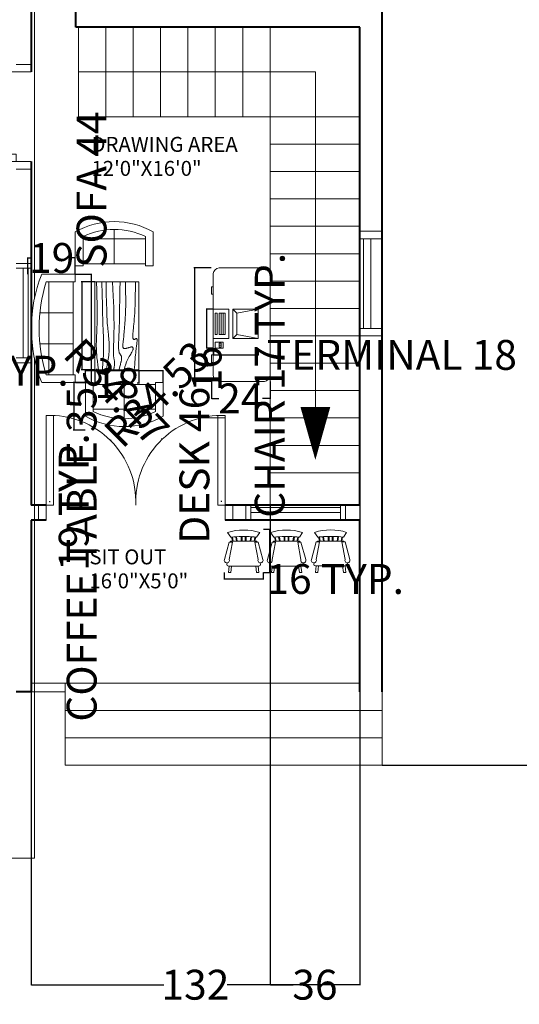
# Model space of a CAD drawing. Units: inches. Extents: x -101 to 786, y 26 to 880.
# Tile 2 of 9: x 178 to 379, y 26 to 422. Entities that reach past the tile are written whole.
import ezdxf

# ---------------------------------------------------------------- set-up
doc = ezdxf.new("R2010")
doc.units = ezdxf.units.IN
doc.header["$MEASUREMENT"] = 0
for name, color, linetype, lineweight in [('A-ANNO-DIMS', 2, 'Continuous', 18), ('A-ANNO-SYMB', 2, 'Continuous', 18), ('A-AREA-IDEN', 7, 'Continuous', 18), ('A-DOOR', 4, 'Continuous', 20), ('A-EQPM', 8, 'Continuous', 13), ('A-FLOR-STRS', 7, 'Continuous', 20), ('A-FURN', 8, 'Continuous', 13), ('A-GLAZ', 4, 'Continuous', 18), ('A-WALL', 7, 'Continuous', 40)]:
    doc.layers.add(name, color=color, linetype=linetype, lineweight=lineweight)
doc.styles.get("Standard").update_dxf_attribs({"font": 'arial.ttf'})
doc.dimstyles.get("Standard").update_dxf_attribs({"dimtxt": 12, "dimasz": 0.18, "dimexe": 0.18, "dimexo": 0.0625, "dimgap": 0.09, "dimtad": 0, "dimdec": 1, "dimzin": 0, "dimdsep": 46, "dimlunit": 3, "dimtxsty": 'Standard', "dimcen": 0.09, "dimadec": 0, "dimazin": 0, "dimtfac": 1, "dimtdec": 1, "dimtofl": 0, "dimtmove": 0, "dimatfit": 3, "dimfxl": 1, "dimtolj": 1, "dimtzin": 0, "dimarcsym": 0})

# ---------------------------------------------------------------- blocks, each defined once
blk = doc.blocks.new('Desk - 30 x 60 in.')
for p, q in [((-26.999995, 0), (26.999995, 0)), ((-29.999995, -27), (-29.999995, -3)), ((29.999995, -3), (29.999995, -27)), ((26.999995, -30), (-26.999995, -30)), ((-20.000005, -30), (-20.000005, -31)), ((-20.000005, -31), (-16.000005, -31)), ((-16.000005, -31), (-16.000005, -30)), ((15.999995, -31), (15.999995, -30)), ((19.999995, -31), (15.999995, -31)), ((19.999995, -30), (19.999995, -31))]:
    blk.add_line(p, q)
for centre, start, end in [((-26.499995, -3.5), 98.1301, 171.8699), ((26.499995, -3.5), 8.130102, 81.8699), ((-26.499995, -26.5), 188.1301, 261.8699), ((26.499995, -26.5), 278.1301, 351.8699)]:
    blk.add_arc(centre, 3.535534, start, end)
blk = doc.blocks.new('Sofa - Roundback 7 ft.')
for p, q in [((-12.00002, -32.4421), (-12.00003, -6.5971)), ((11.99997, -32.4421), (11.99998, -6.5971)), ((-36.000027, -34), (-36.000027, -11.4696)), ((-35.999844, -13.3819), (35.9998, -13.3819)), ((35.99998, -34), (35.99998, -11.4696)), ((-36.000027, -32.4421), (35.99998, -32.4421))]:
    blk.add_line(p, q)
for points in [[(-36.000027, -34), (-42.000027, -34), (-42.000027, -8)], [(41.99998, -8), (41.99998, -34), (35.99998, -34)]]:
    blk.add_lwpolyline(points)
for centre, radius, start, end in [((0, -114.25), 114.25, 68.43141, 111.5686), ((-0.00001, -127.1968), 121.1968, 72.72033, 107.2797)]:
    blk.add_arc(centre, radius, start, end)
blk = doc.blocks.new('Sofa - Roundback Loveseat 5 ft.')
for p, q in [((0, -32.44198), (0, -5.99998)), ((-24, -33.99998), (-24, -11.46958)), ((-23.9998, -13.38178), (23.99986, -13.38178)), ((24.00004, -33.99998), (24.00004, -11.46958)), ((-24, -32.44198), (24.00004, -32.44198))]:
    blk.add_line(p, q)
for points in [[(-24, -33.99998), (-30, -33.99998), (-30, -7.99998)], [(30.00004, -7.99998), (30.00004, -33.99998), (24.00004, -33.99998)]]:
    blk.add_lwpolyline(points)
for centre, radius, start, end in [((0, -60.24998), 60.24998, 60.13715, 119.8628), ((0, -61.38438), 55.38444, 64.32083, 115.6792)]:
    blk.add_arc(centre, radius, start, end)
blk = doc.blocks.new('Table - Rectangular Woodgrain 60 x 30 in.')
for p, q in [((0, 0), (0, -30)), ((60, 0), (0, 0)), ((60, -30), (60, 0)), ((0, -30), (60, -30))]:
    blk.add_line(p, q)
for points in [[(0, -2.4), (4.8155, -2.418), (9.0302, -2.4688), (12.709, -2.5477), (15.9167, -2.65), (18.7181, -2.7711), (21.1781, -2.9063), (23.3616, -3.0508), (25.3333, -3.2), (27.1477, -3.3495), (28.8172, -3.4958), (30.3437, -3.636), (31.7291, -3.7667), (32.9756, -3.8849), (34.0849, -3.9875), (35.059, -4.0714), (35.9, -4.1334), (36.6114, -4.1711), (37.2041, -4.1854), (37.6906, -4.1779), (38.0833, -4.15), (38.3948, -4.1034), (38.6375, -4.0396), (38.8239, -3.9602), (38.9666, -3.8667), (39.0764, -3.7608), (39.1573, -3.6448), (39.2116, -3.521), (39.2416, -3.3917), (39.2498, -3.2593), (39.2385, -3.1261), (39.21, -2.9944), (39.1666, -2.8667), (39.111, -2.7447), (39.0468, -2.6281), (38.978, -2.5163), (38.9083, -2.4083), (38.8418, -2.3035), (38.7823, -2.201), (38.7337, -2.1001), (38.7, -2), (38.6844, -1.9003), (38.6875, -1.8021), (38.7094, -1.707), (38.75, -1.6167), (38.8094, -1.5326), (38.8875, -1.4563), (38.9844, -1.3893), (39.1, -1.3333), (39.2351, -1.2896), (39.3937, -1.2583), (39.5804, -1.2396), (39.8, -1.2333), (40.057, -1.2396), (40.3562, -1.2583), (40.7023, -1.2896), (41.1, -1.3333), (41.5547, -1.3895), (42.0755, -1.4573), (42.6721, -1.5361), (43.3542, -1.625), (44.1316, -1.7233), (45.014, -1.8302), (46.0114, -1.9449), (47.1333, -2.0667), (48.3862, -2.1947), (49.7625, -2.3281), (51.2513, -2.4663), (52.8416, -2.6083), (54.5226, -2.7535), (56.2833, -2.9011), (58.1127, -3.0501), (60, -3.2)], [(0, -9.2), (6.5759, -9.0858), (11.9385, -9.0365), (16.2527, -9.0418), (19.6833, -9.0917), (22.3952, -9.1759), (24.5531, -9.2844), (26.322, -9.4069), (27.8666, -9.5333), (29.3241, -9.6553), (30.7203, -9.7719), (32.0532, -9.8837), (33.3208, -9.9917), (34.5213, -10.0965), (35.6526, -10.199), (36.7128, -10.2999), (37.7, -10.4), (38.6129, -10.4996), (39.4531, -10.5969), (40.223, -10.6895), (40.925, -10.775), (41.5613, -10.8512), (42.1344, -10.9156), (42.6465, -10.966), (43.1, -11), (43.4976, -11.0158), (43.8437, -11.0136), (44.143, -10.9942), (44.4, -10.9583), (44.6195, -10.9069), (44.8062, -10.8406), (44.9648, -10.7603), (45.1, -10.6667), (45.2155, -10.5598), (45.3114, -10.4365), (45.3871, -10.2929), (45.4416, -10.125), (45.4743, -9.929), (45.4844, -9.7011), (45.4709, -9.4371), (45.4333, -9.1333), (45.3716, -8.7883), (45.2896, -8.4104), (45.1919, -8.0107), (45.0833, -7.6), (44.9685, -7.1893), (44.8521, -6.7896), (44.7388, -6.4117), (44.6333, -6.0667), (44.54, -5.7628), (44.4614, -5.4979), (44.4001, -5.2675), (44.3583, -5.0667), (44.3384, -4.8909), (44.3427, -4.7354), (44.3736, -4.5956), (44.4333, -4.4667), (44.5236, -4.3453), (44.6427, -4.2333), (44.7884, -4.1339), (44.9583, -4.05), (45.1501, -3.9849), (45.3614, -3.9417), (45.59, -3.9234), (45.8333, -3.9333), (46.0915, -3.9749), (46.3734, -4.0531), (46.6906, -4.1736), (47.0542, -4.3417), (47.4756, -4.5629), (47.9661, -4.8427), (48.5372, -5.1866), (49.2, -5.6), (49.9676, -6.0844), (50.8594, -6.625), (51.8965, -7.2031), (53.1, -7.8), (54.491, -8.3969), (56.0906, -8.975), (57.9199, -9.5156), (60, -10)], [(0, -12.8), (5.1847, -12.9322), (9.6213, -13.0323), (13.3963, -13.1059), (16.5958, -13.1583), (19.3063, -13.1952), (21.614, -13.2219), (23.6054, -13.2439), (25.3666, -13.2667), (26.9728, -13.2947), (28.4531, -13.3281), (29.8256, -13.3663), (31.1083, -13.4083), (32.3191, -13.4535), (33.476, -13.501), (34.597, -13.5501), (35.7, -13.6), (36.7984, -13.6497), (37.8875, -13.6979), (38.9578, -13.743), (40, -13.7833), (41.0047, -13.8174), (41.9625, -13.8438), (42.864, -13.8607), (43.7, -13.8667), (44.4631, -13.8604), (45.1552, -13.8417), (45.7801, -13.8104), (46.3416, -13.7667), (46.8439, -13.7104), (47.2906, -13.6417), (47.6858, -13.5604), (48.0333, -13.4667), (48.3375, -13.3608), (48.6042, -13.2448), (48.8396, -13.121), (49.05, -12.9917), (49.2417, -12.8593), (49.4208, -12.7261), (49.5937, -12.5944), (49.7667, -12.4667), (49.9452, -12.3451), (50.1323, -12.2313), (50.3303, -12.1268), (50.5416, -12.0333), (50.7686, -11.9524), (51.0135, -11.8854), (51.2788, -11.8341), (51.5666, -11.8), (51.8785, -11.7843), (52.2116, -11.7865), (52.562, -11.8059), (52.926, -11.8417), (53.2998, -11.8931), (53.6795, -11.9594), (54.0614, -12.0397), (54.4416, -12.1333), (54.8223, -12.2401), (55.2293, -12.3625), (55.6942, -12.5037), (56.2489, -12.6667), (56.9251, -12.8547), (57.7545, -13.0708), (58.7689, -13.3182), (60, -13.6)], [(0, -18), (5.124, -17.7273), (9.6609, -17.5057), (13.6705, -17.3303), (17.2125, -17.1958), (20.3467, -17.0973), (23.1328, -17.0297), (25.6307, -16.9878), (27.9, -16.9667), (29.9928, -16.9617), (31.9302, -16.9703), (33.7254, -16.9907), (35.3917, -17.0208), (36.9423, -17.0588), (38.3906, -17.1026), (39.7499, -17.1503), (41.0333, -17.2), (42.2519, -17.2496), (43.4073, -17.2969), (44.4986, -17.3395), (45.525, -17.375), (46.4858, -17.4012), (47.3802, -17.4156), (48.2074, -17.416), (48.9667, -17.4), (49.6583, -17.3662), (50.2872, -17.3167), (50.8595, -17.2547), (51.3812, -17.1833), (51.8584, -17.1057), (52.2971, -17.025), (52.7034, -16.9443), (53.0833, -16.8667), (53.443, -16.7951), (53.789, -16.7313), (54.128, -16.6768), (54.4666, -16.6334), (54.8115, -16.6024), (55.1693, -16.5854), (55.5465, -16.5841), (55.95, -16.6), (56.3828, -16.6337), (56.8346, -16.6823), (57.2915, -16.7418), (57.7396, -16.8084), (58.165, -16.878), (58.5539, -16.9469), (58.8924, -17.0111), (59.1666, -17.0667), (59.3679, -17.1107), (59.5078, -17.1438), (59.6032, -17.1675), (59.6708, -17.1833), (59.7275, -17.193), (59.7901, -17.1979), (59.8753, -17.1998), (60, -17.2)], [(0, -22.4), (8.0098, -22.2501), (14.4094, -22.1011), (19.4168, -21.9535), (23.25, -21.8083), (26.1269, -21.6663), (28.2656, -21.5281), (29.884, -21.3947), (31.2, -21.2667), (32.3967, -21.1448), (33.5172, -21.0292), (34.5697, -20.9198), (35.5625, -20.8167), (36.5037, -20.7198), (37.4015, -20.6292), (38.2642, -20.5448), (39.1, -20.4667), (39.9164, -20.3951), (40.7187, -20.3313), (41.5117, -20.2768), (42.3, -20.2333), (43.0883, -20.2024), (43.8812, -20.1854), (44.6836, -20.1841), (45.5, -20.2), (46.3328, -20.234), (47.1747, -20.2844), (48.0163, -20.3488), (48.8479, -20.425), (49.66, -20.5106), (50.4429, -20.6031), (51.1872, -20.7004), (51.8833, -20.8), (52.5246, -20.8999), (53.1166, -20.9995), (53.6681, -21.0983), (54.1875, -21.1958), (54.6834, -21.2919), (55.1646, -21.3859), (55.6394, -21.4777), (56.1167, -21.5667), (56.6028, -21.6515), (57.0961, -21.7266), (57.5929, -21.7852), (58.0896, -21.8208), (58.5823, -21.8268), (59.0674, -21.7964), (59.5412, -21.723), (60, -21.6)], [(0, -25.2), (8.6355, -25.0504), (15.7026, -24.9031), (21.4049, -24.7606), (25.9458, -24.625), (29.529, -24.4988), (32.3578, -24.3844), (34.6359, -24.284), (36.5667, -24.2), (38.3213, -24.1341), (39.9417, -24.0854), (41.437, -24.0523), (42.8167, -24.0333), (44.0901, -24.0268), (45.2667, -24.0313), (46.3557, -24.0451), (47.3667, -24.0667), (48.309, -24.0947), (49.1928, -24.1287), (50.0284, -24.168), (50.826, -24.2125), (51.5959, -24.2617), (52.3483, -24.3151), (53.0935, -24.3725), (53.8417, -24.4334), (54.6009, -24.497), (55.3699, -24.561), (56.1454, -24.6226), (56.9239, -24.6792), (57.7021, -24.7279), (58.4764, -24.7662), (59.2435, -24.7911), (60, -24.8)], [(0, -28.8), (5.6867, -28.6681), (10.45, -28.5698), (14.407, -28.5012), (17.675, -28.4584), (20.3711, -28.4374), (22.6125, -28.4344), (24.5164, -28.4455), (26.2, -28.4667), (27.762, -28.4947), (29.2276, -28.5281), (30.6033, -28.5663), (31.8958, -28.6084), (33.1118, -28.6535), (34.2578, -28.7011), (35.3405, -28.7501), (36.3666, -28.8), (37.3443, -28.8497), (38.288, -28.8974), (39.2137, -28.9412), (40.1375, -28.9792), (41.0753, -29.0093), (42.0432, -29.0297), (43.0572, -29.0384), (44.1333, -29.0333), (45.2936, -29.0114), (46.5843, -28.9641), (48.0579, -28.8816), (49.7666, -28.7542), (51.7629, -28.5721), (54.0989, -28.3255), (56.8272, -28.0048), (60, -27.6)]]:
    blk.add_lwpolyline(points)
blk = doc.blocks.new('Computer Terminal')
for p, q in [((-10, 11.5), (5, 11.5)), ((-8, 0.5), (-10, 11.5)), ((-10, -1.5), (-10, 11.5)), ((5, 11.5), (3, 0.5)), ((5, 11.5), (5, -1.5)), ((-10, -1.5), (-8, 0.5)), ((3, 0.5), (-8, 0.5)), ((3, 0.5), (5, -1.5)), ((5, -1.5), (-10, -1.5)), ((-10, -11.5), (-10, -3.5)), ((-10, -3.5), (5, -3.5)), ((5, -3.5), (5, -11.5)), ((-8, -5.5), (-8, -8.5)), ((3, -5.5), (-8, -5.5)), ((3, -6.5), (-8, -6.5)), ((-8, -7.5), (3, -7.5)), ((-8, -8.5), (3, -8.5)), ((-8, -9.5), (-8, -10.5)), ((3, -9.5), (-8, -9.5)), ((3, -8.5), (3, -5.5)), ((3, -10.5), (3, -9.5)), ((10, -6.5), (7, -6.5)), ((7, -6.5), (7, -10.5)), ((9.5, -7.5), (7.5, -7.5)), ((7.5, -7.5), (7.5, -8.5)), ((7.5, -8.5), (9.5, -8.5)), ((8.5, -7.5), (8.5, -8.5)), ((9.5, -8.5), (9.5, -7.5)), ((10, -10.5), (10, -6.5)), ((5, -11.5), (-10, -11.5)), ((-8, -10.5), (3, -10.5)), ((7, -10.5), (10, -10.5))]:
    blk.add_line(p, q)
blk = doc.blocks.new('Chair - Rocking')
for p, q in [((-8, -4.5), (-10, -1.5)), ((-7.5, -4.5), (-7, -7)), ((-6.5, -7), (-7.02225, -4.43)), ((-4.5, -7), (-4.96674, -4.19951)), ((-4, -7), (-4.40532, -4.16272)), ((-1.5, -4.05012), (-1.5, -7)), ((-1, -7), (-1, -4.05012)), ((1, -7), (1, -4.04655)), ((1.5, -4.05012), (1.5, -7)), ((4, -7), (4.40187, -4.18694)), ((4.5, -7), (4.96761, -4.19437)), ((6.5, -7), (7, -4.4057)), ((7.5, -4.5), (7, -7)), ((8, -4.5), (10, -1.5)), ((-9, -7.5), (-12, -18.49999)), ((-7, -7.5), (-9, -7.5)), ((-9, -18.49999), (-7, -7.5)), ((-8.23428, -6.99939), (-8.3093, -7.47958)), ((-8.23041, -7), (8.23915, -7)), ((7, -7.5), (9, -7.5)), ((9, -18.49999), (7, -7.5)), ((8.31071, -7.48854), (8.23449, -7.00073)), ((9, -7.5), (12, -18.49999)), ((-10.36644, -20.64523), (-10.5, -21.49999)), ((-9, -22.49999), (-9.5, -26.49999)), ((0, -22.49999), (-9.5, -22.49999)), ((-8, -26.49999), (-7.5, -22.49999)), ((0, -22.49999), (9.5, -22.49999)), ((8, -26.49999), (7.5, -22.49999)), ((9, -22.49999), (9.5, -26.49999)), ((10.5, -21.49999), (10.3575, -20.58798)), ((-9.5, -26.49999), (-8, -26.49999)), ((9.5, -26.49999), (8, -26.49999))]:
    blk.add_line(p, q)
for centre, radius, start, end in [((0, -34.08333), 34.08333, 72.93847, 107.0615), ((0, -68.25004), 64.25, 93.92211, 97.15267), ((0, -68.25004), 64.25, 82.84733, 93.92211), ((-10.5, -18.99999), 1.58114, 161.5651, 18.43495), ((-9.5, -21.49999), 1, 180, 270), ((10.5, -18.99999), 1.58114, 161.5651, 18.43495), ((9.5, -21.49999), 1, 270, 0)]:
    blk.add_arc(centre, radius, start, end)
blk = doc.blocks.new('DOOR-SINGLE-36')
for p, q in [((-39, 0), (-39, -6)), ((-36, 0), (-36, -6)), ((0, 0), (0, -6)), ((3, 0), (3, -6))]:
    blk.add_line(p, q)
blk.add_lwpolyline([(0, 0), (-3, 0), (-3, 36), (0, 36)], close=True)
blk.add_arc((-1.5, 1.5), 34.53, 87.5104, 182.4896)
blk = doc.blocks.new('WIN-36-WALL9')
for p, q in [((0, 42), (9, 42)), ((0, 39), (9, 39)), ((1.5, 39), (1.5, 3)), ((4.5, 39), (4.5, 3)), ((9, 3), (0, 3)), ((9, 0), (0, 0))]:
    blk.add_line(p, q)
blk = doc.blocks.new('*D29')
at = {"layer": 'A-ANNO-DIMS', "color": 0, "lineweight": -2, "transparency": 16777216}
for p, q in [((275.82, 217.12), (278.54, 217.12)), ((278.36, 217.12), (278.36, 217.3)), ((278.36, 199.92), (278.36, 216.94)), ((275.82, 199.74), (278.54, 199.74))]:
    blk.add_line(p, q, dxfattribs=at)
at = {"layer": 'A-ANNO-DIMS', "color": 0, "transparency": 16777216}
for points in [[(278.33, 216.94), (278.39, 216.94), (278.36, 217.12)], [(278.33, 199.92), (278.39, 199.92), (278.36, 199.74)]]:
    blk.add_solid(points, dxfattribs=at)
at = {"layer": 'Defpoints', "color": 0, "transparency": 16777216}
for p in [(275.76, 217.12), (278.36, 217.12), (275.76, 199.74)]:
    blk.add_point(p, dxfattribs=at)
at = {"layer": 'A-ANNO-DIMS', "color": 0, "transparency": 16777216, "insert": (278.36, 274.93), "char_height": 12, "attachment_point": 5, "rotation": 90}
blk.add_mtext('\\A1;CHAIR 17 TYP.', dxfattribs=at)
blk = doc.blocks.new('*D30')
at = {"layer": 'A-ANNO-DIMS', "color": 0, "lineweight": -2, "transparency": 16777216}
for p, q in [((260.03, 199.68), (260.03, 196.96)), ((275.76, 199.68), (275.76, 196.96)), ((260.21, 197.14), (275.58, 197.14)), ((275.76, 197.14), (275.94, 197.14))]:
    blk.add_line(p, q, dxfattribs=at)
at = {"layer": 'A-ANNO-DIMS', "color": 0, "transparency": 16777216}
for points in [[(260.21, 197.17), (260.21, 197.11), (260.03, 197.14)], [(275.58, 197.17), (275.58, 197.11), (275.76, 197.14)]]:
    blk.add_solid(points, dxfattribs=at)
at = {"layer": 'Defpoints', "color": 0, "transparency": 16777216}
for p in [(260.03, 199.74), (275.76, 199.74), (275.76, 197.14)]:
    blk.add_point(p, dxfattribs=at)
at = {"layer": 'A-ANNO-DIMS', "color": 0, "transparency": 16777216, "insert": (304.67, 197.14), "char_height": 12, "attachment_point": 5}
blk.add_mtext('\\A1;16 TYP.', dxfattribs=at)
blk = doc.blocks.new('*D55')
at = {"layer": 'A-ANNO-DIMS', "color": 0, "lineweight": -2, "transparency": 16777216}
for p, q in [((204.29, 276.16), (204.29, 280.97)), ((235.59, 276.16), (235.59, 280.97)), ((204.29, 280.79), (204.11, 280.79)), ((235.41, 280.79), (204.47, 280.79))]:
    blk.add_line(p, q, dxfattribs=at)
at = {"layer": 'A-ANNO-DIMS', "color": 0, "transparency": 16777216}
for points in [[(204.47, 280.82), (204.47, 280.76), (204.29, 280.79)], [(235.41, 280.82), (235.41, 280.76), (235.59, 280.79)]]:
    blk.add_solid(points, dxfattribs=at)
at = {"layer": 'Defpoints', "color": 0, "transparency": 16777216}
for p in [(204.29, 280.79), (204.29, 276.1), (235.59, 276.1)]:
    blk.add_point(p, dxfattribs=at)
at = {"layer": 'A-ANNO-DIMS', "color": 0, "transparency": 16777216, "insert": (128.5, 280.79), "char_height": 12, "attachment_point": 5}
blk.add_mtext('\\A1;LOVESEAT 31 TYP.', dxfattribs=at)
blk = doc.blocks.new('*D56')
at = {"layer": 'A-ANNO-DIMS', "color": 0, "lineweight": -2, "transparency": 16777216}
for p, q in [((204.23, 276.1), (199.42, 276.1)), ((199.6, 275.92), (199.6, 257.15)), ((204.23, 256.97), (199.42, 256.97)), ((199.6, 256.97), (199.6, 256.79))]:
    blk.add_line(p, q, dxfattribs=at)
at = {"layer": 'A-ANNO-DIMS', "color": 0, "transparency": 16777216}
for points in [[(199.57, 275.92), (199.63, 275.92), (199.6, 276.1)], [(199.57, 257.15), (199.63, 257.15), (199.6, 256.97)]]:
    blk.add_solid(points, dxfattribs=at)
at = {"layer": 'Defpoints', "color": 0, "transparency": 16777216}
for p in [(204.29, 276.1), (199.6, 256.97), (204.29, 256.97)]:
    blk.add_point(p, dxfattribs=at)
at = {"layer": 'A-ANNO-DIMS', "color": 0, "transparency": 16777216, "insert": (199.6, 228.06), "char_height": 12, "attachment_point": 5, "rotation": 90}
blk.add_mtext('\\A1;19 TYP.', dxfattribs=at)
blk = doc.blocks.new('*D69')
at = {"layer": 'A-ANNO-DIMS', "color": 0, "lineweight": -2, "transparency": 16777216}
for p, q in [((254.88, 322.12), (247.93, 322.12)), ((248.11, 321.94), (248.11, 276.7)), ((254.88, 276.52), (247.93, 276.52)), ((248.11, 276.52), (248.11, 276.34))]:
    blk.add_line(p, q, dxfattribs=at)
at = {"layer": 'A-ANNO-DIMS', "color": 0, "transparency": 16777216}
for points in [[(248.08, 321.94), (248.14, 321.94), (248.11, 322.12)], [(248.08, 276.7), (248.14, 276.7), (248.11, 276.52)]]:
    blk.add_solid(points, dxfattribs=at)
at = {"layer": 'Defpoints', "color": 0, "transparency": 16777216}
for p in [(254.95, 322.12), (248.11, 276.52), (254.95, 276.52)]:
    blk.add_point(p, dxfattribs=at)
at = {"layer": 'A-ANNO-DIMS', "color": 0, "transparency": 16777216, "insert": (248.11, 242.81), "char_height": 12, "attachment_point": 5, "rotation": 90}
blk.add_mtext('\\A1;DESK 46', dxfattribs=at)
blk = doc.blocks.new('*D70')
at = {"layer": 'A-ANNO-DIMS', "color": 0, "lineweight": -2, "transparency": 16777216}
for p, q in [((254.95, 276.46), (254.95, 269.5)), ((278.51, 276.46), (278.51, 269.5)), ((255.13, 269.68), (257.96, 269.68)), ((278.33, 269.68), (275.49, 269.68))]:
    blk.add_line(p, q, dxfattribs=at)
at = {"layer": 'A-ANNO-DIMS', "color": 0, "transparency": 16777216}
for points in [[(255.13, 269.71), (255.13, 269.65), (254.95, 269.68)], [(278.33, 269.71), (278.33, 269.65), (278.51, 269.68)]]:
    blk.add_solid(points, dxfattribs=at)
at = {"layer": 'Defpoints', "color": 0, "transparency": 16777216}
for p in [(254.95, 276.52), (278.51, 276.52), (278.51, 269.68)]:
    blk.add_point(p, dxfattribs=at)
at = {"layer": 'A-ANNO-DIMS', "color": 0, "transparency": 16777216, "insert": (266.73, 269.68), "char_height": 12, "attachment_point": 5}
blk.add_mtext('\\A1;24', dxfattribs=at)
blk = doc.blocks.new('*D71')
at = {"layer": 'A-ANNO-DIMS', "color": 0, "lineweight": -2, "transparency": 16777216}
for p, q in [((200.31, 319.56), (206.96, 319.56)), ((206.78, 319.56), (206.78, 319.74)), ((206.78, 276.19), (206.78, 319.38)), ((200.31, 276.01), (206.96, 276.01))]:
    blk.add_line(p, q, dxfattribs=at)
at = {"layer": 'A-ANNO-DIMS', "color": 0, "transparency": 16777216}
for points in [[(206.75, 319.38), (206.81, 319.38), (206.78, 319.56)], [(206.75, 276.19), (206.81, 276.19), (206.78, 276.01)]]:
    blk.add_solid(points, dxfattribs=at)
at = {"layer": 'Defpoints', "color": 0, "transparency": 16777216}
for p in [(200.25, 319.56), (206.78, 319.56), (200.25, 276.01)]:
    blk.add_point(p, dxfattribs=at)
at = {"layer": 'A-ANNO-DIMS', "color": 0, "transparency": 16777216, "insert": (206.78, 353.52), "char_height": 12, "attachment_point": 5, "rotation": 90}
blk.add_mtext('\\A1;SOFA 44', dxfattribs=at)
blk = doc.blocks.new('*D72')
at = {"layer": 'A-ANNO-DIMS', "color": 0, "lineweight": -2, "transparency": 16777216}
for p, q in [((181.24, 319.62), (181.24, 326.27)), ((181.42, 326.09), (182.61, 326.09)), ((200.07, 326.09), (198.87, 326.09)), ((200.25, 319.62), (200.25, 326.27))]:
    blk.add_line(p, q, dxfattribs=at)
at = {"layer": 'A-ANNO-DIMS', "color": 0, "transparency": 16777216}
for points in [[(181.42, 326.12), (181.42, 326.06), (181.24, 326.09)], [(200.07, 326.12), (200.07, 326.06), (200.25, 326.09)]]:
    blk.add_solid(points, dxfattribs=at)
at = {"layer": 'Defpoints', "color": 0, "transparency": 16777216}
for p in [(181.24, 326.09), (181.24, 319.56), (200.25, 319.56)]:
    blk.add_point(p, dxfattribs=at)
at = {"layer": 'A-ANNO-DIMS', "color": 0, "transparency": 16777216, "insert": (190.74, 326.09), "char_height": 12, "attachment_point": 5}
blk.add_mtext('\\A1;19', dxfattribs=at)
blk = doc.blocks.new('*D73')
at = {"layer": 'A-ANNO-DIMS', "color": 0, "lineweight": -2, "transparency": 16777216}
for p, q in [((208.06, 316.53), (202.63, 316.53)), ((202.81, 316.35), (202.81, 281.31)), ((208.06, 281.13), (202.63, 281.13)), ((202.81, 281.13), (202.81, 280.95))]:
    blk.add_line(p, q, dxfattribs=at)
at = {"layer": 'A-ANNO-DIMS', "color": 0, "transparency": 16777216}
for points in [[(202.78, 316.35), (202.84, 316.35), (202.81, 316.53)], [(202.78, 281.31), (202.84, 281.31), (202.81, 281.13)]]:
    blk.add_solid(points, dxfattribs=at)
at = {"layer": 'Defpoints', "color": 0, "transparency": 16777216}
for p in [(208.12, 316.53), (202.81, 281.13), (208.12, 281.13)]:
    blk.add_point(p, dxfattribs=at)
at = {"layer": 'A-ANNO-DIMS', "color": 0, "transparency": 16777216, "insert": (202.81, 207.08), "char_height": 12, "attachment_point": 5, "rotation": 90}
blk.add_mtext('\\A1;COFFEE TABLE 35', dxfattribs=at)
blk = doc.blocks.new('*D74')
at = {"layer": 'A-ANNO-DIMS', "color": 0, "lineweight": -2, "transparency": 16777216}
for p, q in [((208.12, 281.06), (208.12, 275.64)), ((225.82, 281.06), (225.82, 275.64)), ((208.3, 275.82), (208.84, 275.82)), ((225.64, 275.82), (225.1, 275.82))]:
    blk.add_line(p, q, dxfattribs=at)
at = {"layer": 'A-ANNO-DIMS', "color": 0, "transparency": 16777216}
for points in [[(208.3, 275.85), (208.3, 275.79), (208.12, 275.82)], [(225.64, 275.85), (225.64, 275.79), (225.82, 275.82)]]:
    blk.add_solid(points, dxfattribs=at)
at = {"layer": 'Defpoints', "color": 0, "transparency": 16777216}
for p in [(208.12, 281.13), (225.82, 281.13), (225.82, 275.82)]:
    blk.add_point(p, dxfattribs=at)
at = {"layer": 'A-ANNO-DIMS', "color": 0, "transparency": 16777216, "insert": (216.97, 275.82), "char_height": 12, "attachment_point": 5}
blk.add_mtext('\\A1;18', dxfattribs=at)
blk = doc.blocks.new('*D75')
at = {"layer": 'A-ANNO-DIMS', "color": 0, "lineweight": -2, "transparency": 16777216}
for p, q in [((255.71, 289.78), (255.71, 286.97)), ((273.71, 289.78), (273.71, 286.97)), ((255.89, 287.15), (273.53, 287.15)), ((273.71, 287.15), (273.89, 287.15))]:
    blk.add_line(p, q, dxfattribs=at)
at = {"layer": 'A-ANNO-DIMS', "color": 0, "transparency": 16777216}
for points in [[(255.89, 287.18), (255.89, 287.12), (255.71, 287.15)], [(273.53, 287.18), (273.53, 287.12), (273.71, 287.15)]]:
    blk.add_solid(points, dxfattribs=at)
at = {"layer": 'Defpoints', "color": 0, "transparency": 16777216}
for p in [(255.71, 289.85), (273.71, 289.85), (273.71, 287.15)]:
    blk.add_point(p, dxfattribs=at)
at = {"layer": 'A-ANNO-DIMS', "color": 0, "transparency": 16777216, "insert": (327.45, 287.15), "char_height": 12, "attachment_point": 5}
blk.add_mtext('\\A1;TERMINAL 18', dxfattribs=at)
blk = doc.blocks.new('*D76')
at = {"layer": 'A-ANNO-DIMS', "color": 0, "lineweight": -2, "transparency": 16777216}
for p, q in [((255.64, 305.5), (252.83, 305.5)), ((253.01, 305.32), (253.01, 290.03)), ((255.64, 289.85), (252.83, 289.85)), ((253.01, 289.85), (253.01, 289.67))]:
    blk.add_line(p, q, dxfattribs=at)
at = {"layer": 'A-ANNO-DIMS', "color": 0, "transparency": 16777216}
for points in [[(252.98, 305.32), (253.04, 305.32), (253.01, 305.5)], [(252.98, 290.03), (253.04, 290.03), (253.01, 289.85)]]:
    blk.add_solid(points, dxfattribs=at)
at = {"layer": 'Defpoints', "color": 0, "transparency": 16777216}
for p in [(255.71, 305.5), (253.01, 289.85), (255.71, 289.85)]:
    blk.add_point(p, dxfattribs=at)
at = {"layer": 'A-ANNO-DIMS', "color": 0, "transparency": 16777216, "insert": (253.01, 281.55), "char_height": 12, "attachment_point": 5, "rotation": 90}
blk.add_mtext('\\A1;16', dxfattribs=at)
blk = doc.blocks.new('*D80')
at = {"layer": 'A-ANNO-DIMS', "color": 0, "lineweight": -2, "transparency": 16777216}
for p, q in [((323.57, 781.8), (424.94, 781.8)), ((424.76, 781.62), (424.76, 472.49)), ((424.76, 122.52), (424.76, 431.66)), ((323.57, 122.34), (424.94, 122.34))]:
    blk.add_line(p, q, dxfattribs=at)
at = {"layer": 'A-ANNO-DIMS', "color": 0, "transparency": 16777216}
for points in [[(424.73, 781.62), (424.79, 781.62), (424.76, 781.8)], [(424.73, 122.52), (424.79, 122.52), (424.76, 122.34)]]:
    blk.add_solid(points, dxfattribs=at)
at = {"layer": 'Defpoints', "color": 0, "transparency": 16777216}
for p in [(323.51, 781.8), (424.76, 781.8), (323.51, 122.34)]:
    blk.add_point(p, dxfattribs=at)
at = {"layer": 'A-ANNO-DIMS', "color": 0, "transparency": 16777216, "insert": (424.76, 452.07), "char_height": 12, "attachment_point": 5, "rotation": 90}
blk.add_mtext('\\A1;659.5', dxfattribs=at)
blk = doc.blocks.new('*D87')
at = {"layer": 'A-ANNO-DIMS', "color": 0, "lineweight": -2, "transparency": 16777216}
for p, q in [((182.51, 155.28), (182.51, 33.98)), ((314.51, 155.28), (314.51, 33.98)), ((182.69, 34.16), (235.79, 34.16)), ((314.33, 34.16), (261.23, 34.16))]:
    blk.add_line(p, q, dxfattribs=at)
at = {"layer": 'A-ANNO-DIMS', "color": 0, "transparency": 16777216}
for points in [[(182.69, 34.19), (182.69, 34.13), (182.51, 34.16)], [(314.33, 34.19), (314.33, 34.13), (314.51, 34.16)]]:
    blk.add_solid(points, dxfattribs=at)
at = {"layer": 'Defpoints', "color": 0, "transparency": 16777216}
for p in [(182.51, 155.34), (314.51, 155.34), (314.51, 34.16)]:
    blk.add_point(p, dxfattribs=at)
at = {"layer": 'A-ANNO-DIMS', "color": 0, "transparency": 16777216, "insert": (248.51, 34.16), "char_height": 12, "attachment_point": 5}
blk.add_mtext('\\A1;132', dxfattribs=at)
blk = doc.blocks.new('*D88')
at = {"layer": 'A-ANNO-DIMS', "color": 0, "lineweight": -2, "transparency": 16777216}
for p, q in [((278.51, 226.74), (278.51, 33.98)), ((314.51, 226.74), (314.51, 33.98)), ((278.69, 34.16), (287.83, 34.16)), ((314.33, 34.16), (305.18, 34.16))]:
    blk.add_line(p, q, dxfattribs=at)
at = {"layer": 'A-ANNO-DIMS', "color": 0, "transparency": 16777216}
for points in [[(278.69, 34.19), (278.69, 34.13), (278.51, 34.16)], [(314.33, 34.19), (314.33, 34.13), (314.51, 34.16)]]:
    blk.add_solid(points, dxfattribs=at)
at = {"layer": 'Defpoints', "color": 0, "transparency": 16777216}
for p in [(278.51, 226.8), (314.51, 226.8), (314.51, 34.16)]:
    blk.add_point(p, dxfattribs=at)
at = {"layer": 'A-ANNO-DIMS', "color": 0, "transparency": 16777216, "insert": (296.51, 34.16), "char_height": 12, "attachment_point": 5}
blk.add_mtext('\\A1;36', dxfattribs=at)
blk = doc.blocks.new('*D131')
at = {"layer": 'A-ANNO-DIMS', "color": 0, "lineweight": -2, "transparency": 16777216}
for p, q in [((214.68, 252.98), (214.55, 252.85)), ((189.92, 228.3), (190.1, 228.3)), ((190.01, 228.21), (190.01, 228.39))]:
    blk.add_line(p, q, dxfattribs=at)
at = {"layer": 'A-ANNO-DIMS', "color": 0, "transparency": 16777216}
blk.add_solid([(214.53, 252.87), (214.57, 252.83), (214.42, 252.72)], dxfattribs=at)
at = {"layer": 'Defpoints', "color": 0, "transparency": 16777216}
for p in [(214.42, 252.72), (190.01, 228.3)]:
    blk.add_point(p, dxfattribs=at)
at = {"layer": 'A-ANNO-DIMS', "color": 0, "transparency": 16777216, "insert": (233.12, 271.42), "char_height": 12, "attachment_point": 5, "rotation": 45.0009}
blk.add_mtext('\\A1;R34.53', dxfattribs=at)
blk = doc.blocks.new('*D132')
at = {"layer": 'A-ANNO-DIMS', "color": 0, "lineweight": -2, "transparency": 16777216}
for p, q in [((234.9, 253.5), (235.02, 253.37)), ((258.92, 228.37), (259.1, 228.37)), ((259.01, 228.28), (259.01, 228.46))]:
    blk.add_line(p, q, dxfattribs=at)
at = {"layer": 'A-ANNO-DIMS', "color": 0, "transparency": 16777216}
blk.add_solid([(235.04, 253.39), (235, 253.35), (235.15, 253.24)], dxfattribs=at)
at = {"layer": 'Defpoints', "color": 0, "transparency": 16777216}
for p in [(235.15, 253.24), (259.01, 228.37)]:
    blk.add_point(p, dxfattribs=at)
at = {"layer": 'A-ANNO-DIMS', "color": 0, "transparency": 16777216, "insert": (216.85, 272.32), "char_height": 12, "attachment_point": 5, "rotation": 313.8063}
blk.add_mtext('\\A1;R34.47', dxfattribs=at)

msp = doc.modelspace()

# ---------------------------------------------------------------- linework, layer by layer
at = {"layer": 'A-ANNO-SYMB'}
for p, q in [((183.8117, 802.4238), (183.8117, 309.6043)), ((183.8117, 285.9621), (183.8117, 84.9238)), ((183.8117, 84.9238), (137.8117, 84.9238))]:
    msp.add_line(p, q, dxfattribs=at)
at = {"layer": 'A-DOOR'}
for p, q in [((260.5071, 261.8033), (250.6333, 261.8033)), ((185.5071, 226.8033), (185.5071, 220.8033)), ((188.5071, 226.8033), (188.5071, 220.8033)), ((260.5071, 226.8033), (260.5071, 220.8033)), ((263.5071, 226.8033), (263.5071, 220.8033))]:
    msp.add_line(p, q, dxfattribs=at)
for points in [[(188.5071, 226.8033), (191.5071, 226.8033), (191.5071, 262.8033), (188.5071, 262.8033)], [(260.5071, 226.8033), (257.5071, 226.8033), (257.5071, 262.8033), (260.5071, 262.8033)]]:
    msp.add_lwpolyline(points, close=True, dxfattribs=at)
for centre, radius, start, end in [((190.0071, 228.3033), 34.5326, 357.510447, 92.489553), ((259.0071, 228.3685), 34.4675, 87.50574, 180.108361)]:
    msp.add_arc(centre, radius, start, end, dxfattribs=at)
at = {"layer": 'A-FLOR-STRS'}
for p, q in [((201.5071, 382.8033), (201.5071, 418.8033)), ((212.5071, 382.8033), (212.5071, 418.8033)), ((223.5071, 382.8033), (223.5071, 418.8033)), ((234.5071, 382.8033), (234.5071, 418.8033)), ((245.5071, 382.8033), (245.5071, 418.8033)), ((256.5071, 382.8033), (256.5071, 418.8033)), ((267.5071, 382.8033), (267.5071, 418.8033)), ((278.5071, 226.8033), (278.5071, 418.8033)), ((314.5071, 382.8033), (201.5071, 382.8033)), ((314.5071, 371.8033), (278.5071, 371.8033)), ((314.5071, 360.8033), (278.5071, 360.8033)), ((314.5071, 349.8033), (278.5071, 349.8033)), ((314.5071, 338.8033), (278.5071, 338.8033)), ((314.5071, 327.8033), (278.5071, 327.8033)), ((314.5071, 316.8033), (278.5071, 316.8033)), ((314.5071, 305.8033), (278.5071, 305.8033)), ((314.5071, 294.8033), (278.5071, 294.8033)), ((314.5071, 283.8033), (278.5071, 283.8033)), ((314.5071, 272.8033), (278.5071, 272.8033)), ((314.5071, 261.8033), (278.5071, 261.8033)), ((314.5071, 250.8033), (278.5071, 250.8033)), ((314.5071, 239.8033), (278.5071, 239.8033)), ((196.1887, 155.3446), (182.5071, 155.3446)), ((196.1887, 155.3446), (314.5071, 155.3446)), ((196.1887, 155.3446), (196.1887, 122.3446)), ((196.1887, 122.3446), (196.1887, 155.3446)), ((314.5071, 155.3446), (314.5071, 144.3446)), ((182.5071, 151.8033), (196.1887, 151.8033)), ((323.5071, 151.8033), (323.5071, 122.3446)), ((196.1887, 144.3446), (323.5071, 144.3446)), ((196.1887, 133.3446), (323.5071, 133.3446)), ((196.1887, 122.3446), (323.5071, 122.3446))]:
    msp.add_line(p, q, dxfattribs=at)
msp.add_lwpolyline([(201.5071, 400.8033), (296.7012, 400.8033), (296.7012, 266.2483)], dxfattribs=at)
msp.add_lwpolyline([(296.7012, 266.2483, 12, 0, 0), (296.7012, 244.9541, 0, 0, 0)], format="xyseb", dxfattribs=at)
at = {"layer": 'A-GLAZ'}
for p, q in [((182.5071, 323.9238), (176.5071, 323.9238)), ((182.5071, 321.9238), (176.5071, 321.9238)), ((179.3117, 285.9238), (179.3117, 321.9238)), ((181.3117, 285.9238), (181.3117, 321.9238)), ((176.5071, 285.9238), (182.5071, 285.9238)), ((176.5071, 283.9238), (182.5071, 283.9238)), ((268.8117, 226.8033), (268.8117, 220.8033)), ((270.8117, 226.8033), (270.8117, 220.8033)), ((270.8117, 225.8033), (306.8117, 225.8033)), ((306.8117, 220.8033), (306.8117, 226.8033)), ((308.8117, 220.8033), (308.8117, 226.8033)), ((270.8117, 223.8033), (306.8117, 223.8033))]:
    msp.add_line(p, q, dxfattribs=at)
at = {"layer": 'A-WALL'}
for p, q in [((182.5071, 562.8033), (182.5071, 418.8033)), ((200.5071, 418.8033), (200.5071, 562.8033)), ((182.5071, 418.8033), (182.5071, 400.8033)), ((314.5071, 418.8033), (200.5071, 418.8033)), ((314.5071, 226.8033), (314.5071, 418.8033)), ((182.5071, 364.8033), (182.5071, 226.8033)), ((188.5071, 226.8033), (182.5071, 226.8033)), ((314.5071, 226.8033), (260.5071, 226.8033)), ((182.5071, 220.8033), (182.5071, 151.8033)), ((188.5071, 220.8033), (182.5071, 220.8033)), ((314.5071, 220.8033), (260.5071, 220.8033)), ((314.5071, 151.8033), (314.5071, 220.8033)), ((182.5071, 151.8033), (176.5071, 151.8033))]:
    msp.add_line(p, q, dxfattribs=at)
msp.add_lwpolyline([(323.5071, 151.8033), (323.5071, 781.8033), (23.5071, 781.8033), (23.5071, 151.8033)], dxfattribs=at)

# ---------------------------------------------------------------- block references
at = {"layer": 'A-DOOR', "extrusion": (0, 0, -1), "zscale": -1, "rotation": 270.0000000000001}
msp.add_blockref('DOOR-SINGLE-36', (-176.5071, 364.8033), dxfattribs=at)
at = {"layer": 'A-EQPM', "xscale": 0.7828989296344805, "yscale": 0.7828989296344805, "zscale": 0.7828989296344805, "rotation": 270}
msp.add_blockref('Computer Terminal', (264.7096, 297.6759), dxfattribs=at)
at = {"layer": 'A-FURN'}
for name, p, xscale, yscale, zscale in [('Sofa - Roundback Loveseat 5 ft.', (215.8953, 340.6879), 0.521585550133869, 0.521585550133869, 0.521585550133869), ('Chair - Rocking', (267.8953, 216.7988), 0.6435431877562627, 0.6435431877562627, 0.6435431877562627), ('Chair - Rocking', (285.1292, 216.7988), 0.6435431877562627, 0.6435431877562627, 0.6435431877562627), ('Chair - Rocking', (302.8344, 216.8313), 0.6435431877562627, 0.6435431877562627, 0.6435431877562627)]:
    msp.add_blockref(name, p, dxfattribs=dict(at, xscale=xscale, yscale=yscale, zscale=zscale))
for name, p, xscale, yscale, zscale, rotation in [('Desk - 30 x 60 in.', (278.5071, 299.3241), 0.7600282315072326, 0.7600282315072326, 0.7600282315072326, 270), ('Sofa - Roundback 7 ft.', (182.6202, 297.7832), 0.5184569035944397, 0.5184569035944397, 0.5184569035944397, 90), ('Table - Rectangular Woodgrain 60 x 30 in.', (225.8216, 316.5288), 0.590039911196395, 0.590039911196395, 0.590039911196395, 270), ('Sofa - Roundback Loveseat 5 ft.', (219.9402, 258.3628), 0.521585550133869, 0.521585550133869, 0.521585550133869, 180)]:
    msp.add_blockref(name, p, dxfattribs=dict(at, xscale=xscale, yscale=yscale, zscale=zscale, rotation=rotation))
at = {"layer": 'A-GLAZ'}
msp.add_blockref('WIN-36-WALL9', (314.507, 294.8033), dxfattribs=at)

# ---------------------------------------------------------------- texts
at = {"layer": 'A-AREA-IDEN'}
for s, p in [('DRAWING AREA', (206.7483, 368.7071)), ('12\'0"X16\'0"', (206.7483, 359.0687)), ('SIT OUT', (205.9156, 203.0153)), ('16\'0"X5\'0"', (205.9156, 193.3769))]:
    msp.add_text(s, height=6, dxfattribs=at).set_placement(p)

# ---------------------------------------------------------------- dimensions: what is measured, and where the dimension line sits
at = {"layer": 'A-ANNO-DIMS'}
for base, p1, p2, angle, override, picture, middle in [((424.7579, 781.8033), (323.5071, 122.3446), (323.5071, 781.8033), 90, {"dimdec": 1, "dimlfac": 1, "dimrnd": 0, "dimzin": 0, "dimdsep": 46, "dimlunit": 2}, '*D80', (424.7579, 452.0739)), ((181.2376, 326.091), (200.2477, 319.5584), (181.2376, 319.5584), 180, {"dimdec": 0, "dimlfac": 1, "dimrnd": 0, "dimzin": 0, "dimdsep": 46, "dimlunit": 2}, '*D72', (190.7427, 326.091)), ((253.0052, 289.8469), (255.7062, 305.5049), (255.7062, 289.8469), 270, {"dimdec": 0, "dimlfac": 1, "dimrnd": 0, "dimzin": 0, "dimdsep": 46, "dimlunit": 2}, '*D76', (253.0052, 281.551))]:
    dim = msp.add_linear_dim(base=base, p1=p1, p2=p2, angle=angle, dimstyle='Standard', override=override, dxfattribs=at)
    dim.commit()
    dim.dimension.update_dxf_attribs({"geometry": picture, "text_midpoint": middle})
for base, p1, p2, angle, text, picture, middle in [((206.7803, 319.5584), (200.2477, 276.008), (200.2477, 319.5584), 90, 'SOFA <>', '*D71', (206.7803, 353.5201)), ((278.3641, 217.1206), (275.7578, 199.7449), (275.7578, 217.1206), 90, 'CHAIR <> TYP.', '*D29', (278.3641, 274.9349)), ((248.1059, 276.5232), (254.9462, 322.1249), (254.9462, 276.5232), 270, 'DESK <>', '*D69', (248.1059, 242.8071)), ((202.8101, 281.1264), (208.1204, 316.5288), (208.1204, 281.1264), 270, 'COFFEE TABLE <>', '*D73', (202.8101, 207.0801)), ((204.2926, 280.791), (235.5878, 276.0967), (204.2926, 276.0967), 180, 'LOVESEAT <> TYP.', '*D55', (128.4988, 280.791)), ((199.5984, 256.9719), (204.2926, 276.0967), (204.2926, 256.9719), 270, '<> TYP.', '*D56', (199.5984, 228.0607))]:
    dim = msp.add_linear_dim(base=base, p1=p1, p2=p2, angle=angle, text=text, dimstyle='Standard', override={"dimdec": 0, "dimlfac": 1, "dimrnd": 0, "dimzin": 0, "dimdsep": 46, "dimlunit": 2}, dxfattribs=at)
    dim.commit()
    dim.dimension.update_dxf_attribs({"geometry": picture, "text_midpoint": middle})
for base, p1, p2, text, picture, middle in [((273.7129, 287.1459), (255.7062, 289.8469), (273.7129, 289.8469), 'TERMINAL <>', '*D75', (327.4509, 287.1459)), ((275.7578, 197.1386), (260.0327, 199.7449), (275.7578, 199.7449), '<> TYP.', '*D30', (304.669, 197.1386))]:
    dim = msp.add_linear_dim(base=base, p1=p1, p2=p2, text=text, dimstyle='Standard', override={"dimdec": 0, "dimlfac": 1, "dimrnd": 0, "dimzin": 0, "dimdsep": 46, "dimlunit": 2}, dxfattribs=at)
    dim.commit()
    dim.dimension.update_dxf_attribs({"geometry": picture, "text_midpoint": middle})
for center, mpoint, picture, middle in [((190.0071, 228.3033), (214.4249, 252.7219), '*D131', (233.1199, 271.4175)), ((259.0071, 228.3685), (235.1479, 253.2431), '*D132', (216.8462, 272.3238))]:
    dim = msp.add_radius_dim(center=center, mpoint=mpoint, dimstyle='Standard', override={"dimdec": 2, "dimlfac": 1, "dimrnd": 0, "dimzin": 0, "dimdsep": 46, "dimlunit": 2}, dxfattribs=at)
    dim.commit()
    dim.dimension.update_dxf_attribs({"geometry": picture, "text_midpoint": middle})
for base, p1, p2, picture, middle in [((225.8216, 275.816), (208.1204, 281.1264), (225.8216, 281.1264), '*D74', (216.971, 275.816)), ((278.5071, 269.683), (254.9462, 276.5232), (278.5071, 276.5232), '*D70', (266.7266, 269.683)), ((314.5071, 34.1619), (278.5071, 226.8033), (314.5071, 226.8033), '*D88', (296.5071, 34.1619)), ((314.5071, 34.1619), (182.5071, 155.3446), (314.5071, 155.3446), '*D87', (248.5071, 34.1619))]:
    dim = msp.add_linear_dim(base=base, p1=p1, p2=p2, dimstyle='Standard', override={"dimdec": 0, "dimlfac": 1, "dimrnd": 0, "dimzin": 0, "dimdsep": 46, "dimlunit": 2}, dxfattribs=at)
    dim.commit()
    dim.dimension.update_dxf_attribs({"geometry": picture, "text_midpoint": middle})

doc.saveas('drawing.dxf')
